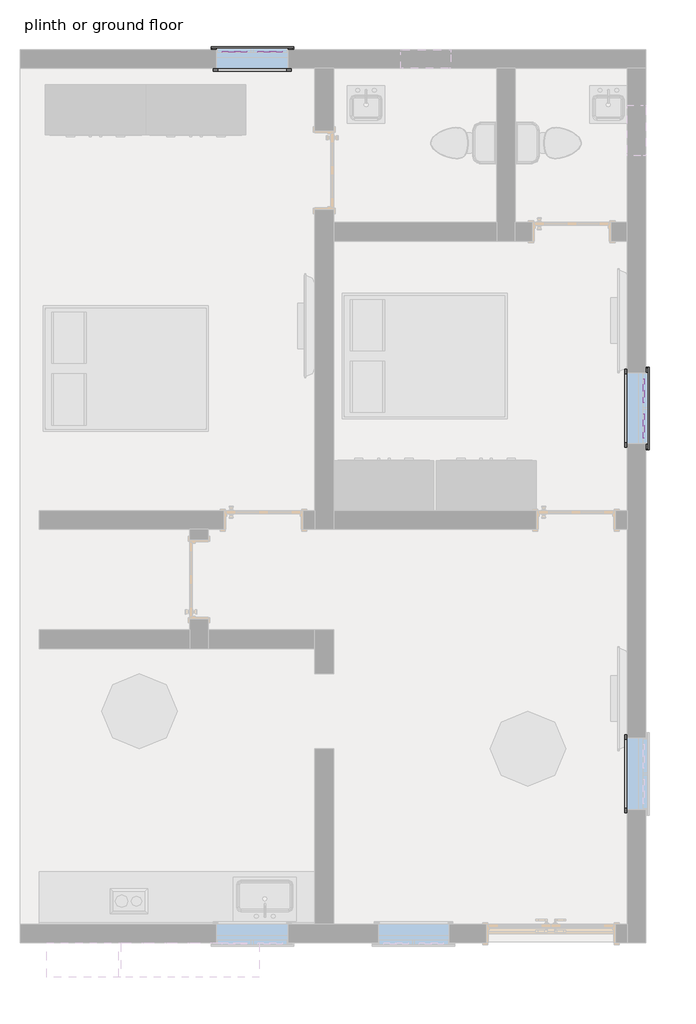
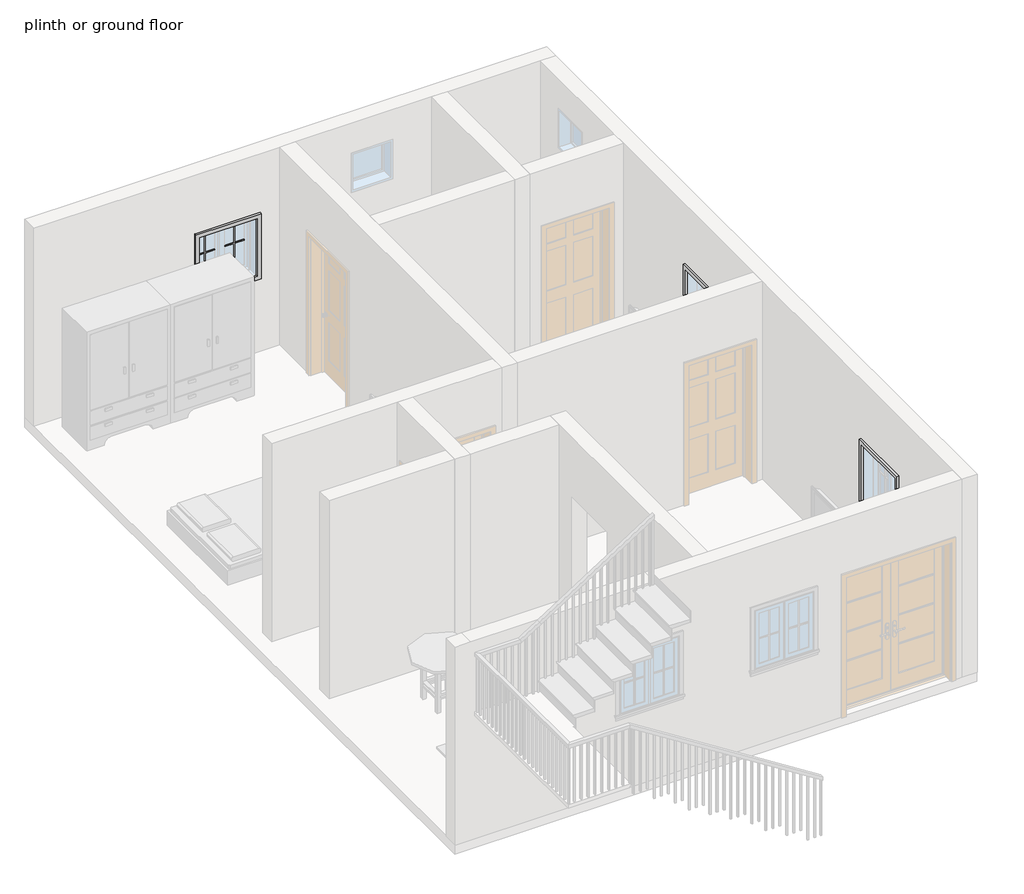
# One storey, part 3 of 3: 9 proxies.
"""IFC4 building model written with IfcOpenShell, lengths in millimetres."""

from ifc_helpers import new_model, si_unit, origin, place, context, project, spatial, transform, mapped, element, save
from components import muntin_pattern_2x2_muntin_pattern_2x2_b3fe6957, muntin_pattern_2x2_muntin_pattern_2x2_3e0ecaf2, trim_window_exterior_flat_with_sill_41619996, trim_window_interior_flat_picture_frame_51c85655

model = new_model("IFC4")

# Units and contexts
model_context = context("Model", 3, world=origin())
ifc_project = project(units=[si_unit("LENGTHUNIT", "METRE", prefix="MILLI")], contexts=[model_context])

# Site, building, storey
site = spatial("IfcSite", under=ifc_project)
building = spatial("IfcBuilding", under=site)
storey = spatial("IfcBuildingStorey", under=building, Name="plinth or ground floor", Elevation=609.6)

# Proxies
placement = place(None, origin())
muntin_pattern_2x2_muntin_pattern_2x2_shape = muntin_pattern_2x2_muntin_pattern_2x2_b3fe6957(model_context)
element("IfcBuildingElementProxy", 1, Name="Muntin Pattern_2x2 : Muntin Pattern_2x2", ObjectType="Muntin Pattern_2x2 : Muntin Pattern_2x2", at=placement, inside=storey, context=model_context, shape_type="MappedRepresentation", body=[
    mapped(muntin_pattern_2x2_muntin_pattern_2x2_shape, transform((26611.0886801, 13049.7534313, 1863.725), x_axis=(0.0, -1.0, 0.0), y_axis=(1.0, 0.0, 0.0), z_axis=(0.0, 0.0, 1.0))),
])
element("IfcBuildingElementProxy", 2, Name="Muntin Pattern_2x2 : Muntin Pattern_2x2", ObjectType="Muntin Pattern_2x2 : Muntin Pattern_2x2", at=placement, inside=storey, context=model_context, shape_type="MappedRepresentation", body=[
    mapped(muntin_pattern_2x2_muntin_pattern_2x2_shape, transform((21618.4011801, 17187.2502787, 1863.725), x_axis=(1.0, 0.0, 0.0), y_axis=(0.0, 1.0, 0.0), z_axis=(0.0, 0.0, 1.0))),
])
muntin_pattern_2x2_muntin_pattern_2x2_2_shape = muntin_pattern_2x2_muntin_pattern_2x2_3e0ecaf2(model_context)
element("IfcBuildingElementProxy", 3, Name="Muntin Pattern_2x2 : Muntin Pattern_2x2", ObjectType="Muntin Pattern_2x2 : Muntin Pattern_2x2", at=placement, inside=storey, context=model_context, shape_type="MappedRepresentation", body=[
    mapped(muntin_pattern_2x2_muntin_pattern_2x2_2_shape, transform((26611.0886801, 12621.1284313, 1863.725), x_axis=(0.0, 1.0, 0.0), y_axis=(-1.0, 0.0, 0.0), z_axis=(0.0, 0.0, 1.0))),
])
element("IfcBuildingElementProxy", 4, Name="Muntin Pattern_2x2 : Muntin Pattern_2x2", ObjectType="Muntin Pattern_2x2 : Muntin Pattern_2x2", at=placement, inside=storey, context=model_context, shape_type="MappedRepresentation", body=[
    mapped(muntin_pattern_2x2_muntin_pattern_2x2_2_shape, transform((22047.0261801, 17187.2502787, 1863.725), x_axis=(-1.0, 0.0, 0.0), y_axis=(0.0, -1.0, 0.0), z_axis=(0.0, 0.0, 1.0))),
])
trim_window_exterior_flat_with_sill_shape = trim_window_exterior_flat_with_sill_41619996(model_context)
element("IfcBuildingElementProxy", 5, Name="Trim-Window-Exterior-Flat : with Sill", ObjectType="Trim-Window-Exterior-Flat : with Sill", at=placement, inside=storey, context=model_context, shape_type="MappedRepresentation", body=[
    mapped(trim_window_exterior_flat_with_sill_shape, transform((26620.6136801, 12835.4409313, 2708.275), x_axis=(0.0, 1.0, 0.0), y_axis=(0.0, 0.0, 1.0), z_axis=(1.0, 0.0, 0.0))),
])
element("IfcBuildingElementProxy", 6, Name="Trim-Window-Exterior-Flat : with Sill", ObjectType="Trim-Window-Exterior-Flat : with Sill", at=placement, inside=storey, context=model_context, shape_type="MappedRepresentation", body=[
    mapped(trim_window_exterior_flat_with_sill_shape, transform((21832.7136801, 17196.7752787, 2708.275), x_axis=(-1.0, 0.0, 0.0), y_axis=(0.0, 0.0, 1.0), z_axis=(0.0, 1.0, 0.0))),
])
trim_window_interior_flat_picture_frame_shape = trim_window_interior_flat_picture_frame_51c85655(model_context)
element("IfcBuildingElementProxy", 7, Name="Trim-Window-Interior-Flat : Picture Frame", ObjectType="Trim-Window-Interior-Flat : Picture Frame", at=placement, inside=storey, context=model_context, shape_type="MappedRepresentation", body=[
    mapped(trim_window_interior_flat_picture_frame_shape, transform((26392.0136801, 12835.4409313, 2708.275), x_axis=(0.0, -1.0, 0.0), y_axis=(0.0, 0.0, 1.0), z_axis=(-1.0, 0.0, 0.0))),
])
element("IfcBuildingElementProxy", 8, Name="Trim-Window-Interior-Flat : Picture Frame", ObjectType="Trim-Window-Interior-Flat : Picture Frame", at=placement, inside=storey, context=model_context, shape_type="MappedRepresentation", body=[
    mapped(trim_window_interior_flat_picture_frame_shape, transform((26392.0136801, 8390.4409313, 2708.275), x_axis=(0.0, -1.0, 0.0), y_axis=(0.0, 0.0, 1.0), z_axis=(-1.0, 0.0, 0.0))),
])
element("IfcBuildingElementProxy", 9, Name="Trim-Window-Interior-Flat : Picture Frame", ObjectType="Trim-Window-Interior-Flat : Picture Frame", at=placement, inside=storey, context=model_context, shape_type="MappedRepresentation", body=[
    mapped(trim_window_interior_flat_picture_frame_shape, transform((21832.7136801, 16968.1752787, 2708.275), x_axis=(1.0, 0.0, 0.0), y_axis=(0.0, 0.0, 1.0), z_axis=(0.0, -1.0, 0.0))),
])

save(model, "model.ifc")

# Revit data of these elements
# Type "Muntin Pattern_2x2 : Muntin Pattern_2x2"
#   Width [instance default] = 4' - 0"
#   Thickness = 0' - 0 1/2"
#   Height [instance default] = 4' - 0"
#   Distance = 0' - 0 3/4"
#   Interior Material [instance default] = none
#   Exterior Material [instance default] = none
#   Default Elevation = 0
# Type "Trim-Window-Exterior-Flat : with Sill"
#   Trim Width = 0' - 2 1/4"
#   Trim Thickness_Picture Frame = 0' - 1 1/4"
#   Trim Thickness_with Sill = 0' - 0 3/4"
#   Sill Thickness = 0' - 1 1/4"
#   Opening Width [instance default] = 2' - 0"
#   Opening Height [instance default] = 3' - 0"
#   Default Elevation = 4' - 0"
#   Sill = yes
#   Picture Frame = no
#   Trim Material [instance default] = none
# Type "Trim-Window-Interior-Flat : Picture Frame"
#   Trim Thickness_Picture Frame = 0' - 1 1/4"
#   Trim Width = 0' - 2 1/4"
#   Trim Thickness_with Sill = 0' - 0 3/4"
#   Sill Thickness = 0' - 1 1/4"
#   Opening Width [instance default] = 2' - 0"
#   Opening Height [instance default] = 3' - 0"
#   Default Elevation = 4' - 0"
#   Sill = no
#   Picture Frame = yes
#   Trim Material [instance default] = none
# Elements 1, 2, 3, 4 (IfcBuildingElementProxy, "Muntin Pattern_2x2 : Muntin Pattern_2x2")
#   Width = 0' - 11 5/8"
#   Height = 2' - 6 1/2"
#   Interior Material = Wood - Stained
#   Exterior Material = Clad - White
#   Phase Created = New Construction
#   Materials on its faces: "Clad - White", "Wood - Stained"
# Elements 5, 6 (IfcBuildingElementProxy, "Trim-Window-Exterior-Flat : with Sill")
#   Opening Width = 2' - 10"
#   Opening Height = 3' - 0"
#   Trim Material = Clad - White
#   Phase Created = New Construction
#   Materials on its faces: "Clad - White"
# Elements 7, 8, 9 (IfcBuildingElementProxy, "Trim-Window-Interior-Flat : Picture Frame")
#   Opening Width = 2' - 10"
#   Opening Height = 3' - 0"
#   Trim Material = Wood - Stained
#   Phase Created = New Construction
#   Materials on its faces: "Wood - Stained"
# Materials
#   "Clad - White": class "Wood", colour RGB 242 242 238, transparency 0, Cost = 0
#   "Wood - Stained": class "Wood", colour RGB 224 178 126, transparency 0, Cost = 0
